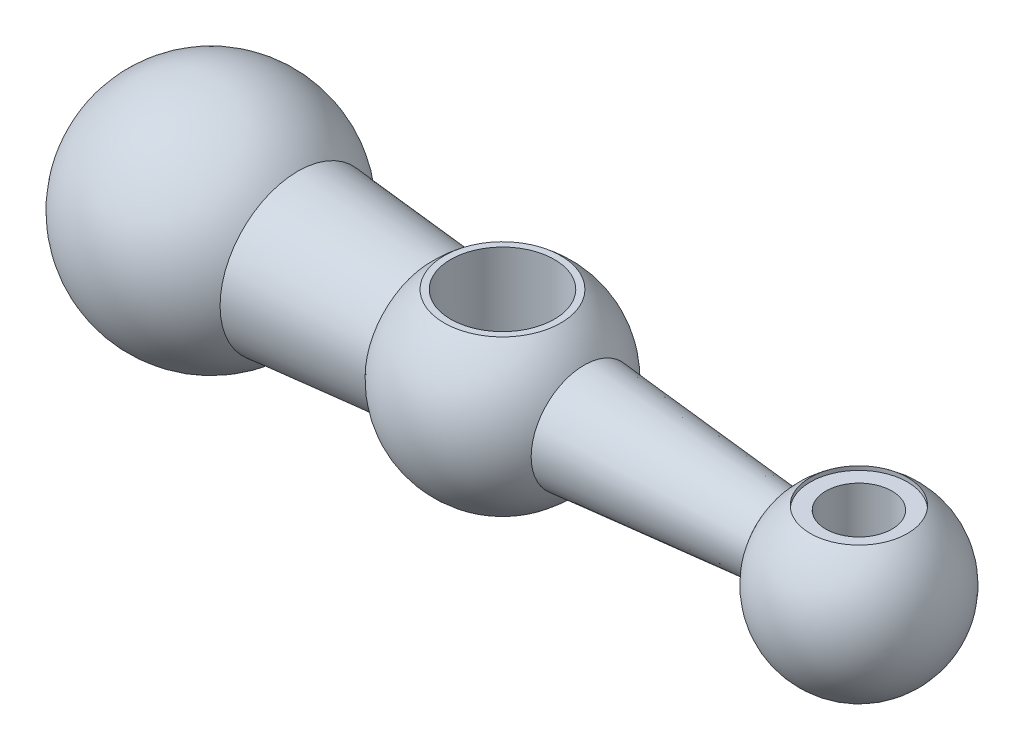
from build123d import *

# Parameters (mm, degrees)
BORE_13_DEPTH                     = 73.608539443
BORE_13_DEPTH_BACK                = 73.608539443
BORE_13_SKETCH_R                  = 8
RECESS_START                      = 10
RECESS_15_SKETCH_R                = 7.5
RECESS_15X10_DEPTH                = 63.608539443
COUNTERBORE_START                 = 12
COUNTERBORE_18_SKETCH_R           = 9
COUNTERBORE_18X12_DEPTH           = 61.608539443
HANDLE_SHANK_BORE_10_2_DEPTH      = 73.608539443
HANDLE_SHANK_BORE_10_2_DEPTH_BACK = 73.608539443
SKETCH6_R                         = 5.1


with BuildPart() as part:
    # Handle Profile Sketch → Handle Body Revolve (revolve)
    with BuildSketch(Plane.XY):
        with BuildLine():
            Line((-31.583592135, 12), (-10.988504472, 10.210424549))
            ThreePointArc((-10.988504472, 10.210424549), (1.298506798, 14.943690311), (12.58494961, 8.162048965))
            Line((12.58494961, 8.162048965), (43.220781011, 5.5))
            ThreePointArc((43.220781011, 5.5), (57.816926795, 12.691135624), (68, 0))
            Line((68, 0), (-63, 0))
            ThreePointArc((-63, 0), (-51.422797616, 16.815102461), (-31.583592135, 12))
        make_face()
    revolve(axis=Axis((-65.491317505, 0, 0), (1, 0, 0)))

    # Bore Ø13 Sketch → Bore Ø13 (cut, two sides: drawn at the far end of the back side and taken through both)
    with BuildSketch(Plane(origin=(0, 0, 0), x_dir=(1, 0, 0), z_dir=(0, 1, 0)).offset(-BORE_13_DEPTH_BACK)):
        with Locations(Location((0, 0, 0), (0, 0, 270))):
            Circle(BORE_13_SKETCH_R)
    extrude(amount=BORE_13_DEPTH + BORE_13_DEPTH_BACK, mode=Mode.SUBTRACT)

    # Recess Ø15 Sketch → Recess Ø15x10 (cut, through all)
    with BuildSketch(Plane(origin=(0, 0, 0), x_dir=(1, 0, 0), z_dir=(0, 1, 0)).offset(RECESS_START)):
        with Locations(Location((55, 0, 0), (0, 0, 90))):
            Circle(RECESS_15_SKETCH_R)
    extrude(amount=RECESS_15X10_DEPTH, mode=Mode.SUBTRACT)

    # Counterbore Ø18 Sketch → Counterbore Ø18x12 (cut, through all)
    with BuildSketch(Plane(origin=(0, 0, 0), x_dir=(1, 0, 0), z_dir=(0, 1, 0)).offset(COUNTERBORE_START)):
        Circle(COUNTERBORE_18_SKETCH_R)
    counterbore_18x12 = extrude(amount=COUNTERBORE_18X12_DEPTH, mode=Mode.SUBTRACT)

    # Counterbore Mirror: Counterbore Ø18x12 across plane
    add(counterbore_18x12.mirror(Plane.ZX), mode=Mode.SUBTRACT)

    # Sketch6 → Handle Shank Bore Ø10.2 (cut, two sides: drawn at the far end of the back side and taken through both)
    with BuildSketch(Plane(origin=(0, 0, 0), x_dir=(1, 0, 0), z_dir=(0, 1, 0)).offset(-HANDLE_SHANK_BORE_10_2_DEPTH_BACK)):
        with Locations(Location((55, 0, 0), (0, 0, 270))):
            Circle(SKETCH6_R)
    extrude(amount=HANDLE_SHANK_BORE_10_2_DEPTH + HANDLE_SHANK_BORE_10_2_DEPTH_BACK, mode=Mode.SUBTRACT)


solid = part.part
